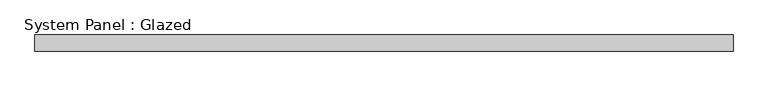
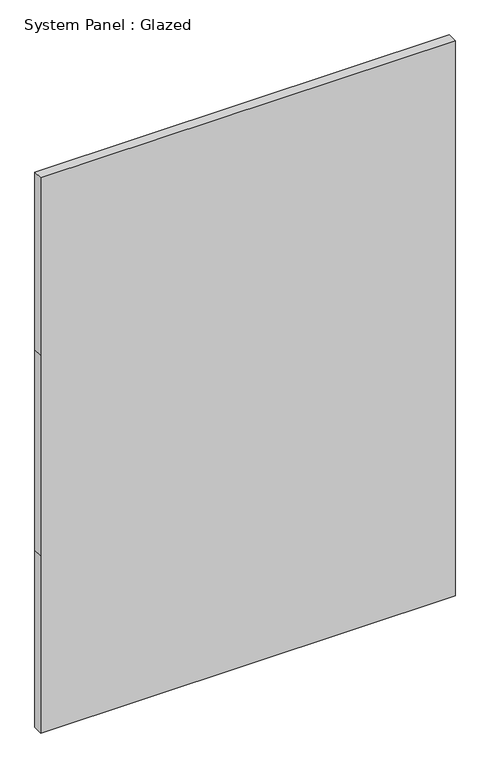
"""IFC4 building model written with IfcOpenShell, lengths in millimetres: plate geometry, System Panel : Glazed."""

from ifc_helpers import new_model, si_unit, frame, origin, place, context, project, spatial, polyline, outline, extrude, source, transform, mapped, element, save


def system_panel_glazed_ce1b7c8d(model_context):
    return source(origin(), model_context, "Body", "SweptSolid", [
        extrude(outline(polyline([(0.0, -536.575), (0.0, 536.575), (485.536674, 536.575), (1034.5733481, 536.575), (1520.1100221, 536.575), (1520.1100221, -536.575), (1034.5733481, -536.575), (485.536674, -536.575), (0.0, -536.575)])), frame((0.0, 19.05, 0.0), z_axis=(0.0, 1.0, 0.0), x_axis=(0.0, 0.0, 1.0)), (0.0, 0.0, 1.0), 25.4),
    ])


if __name__ == "__main__":
    model = new_model("IFC4")
    model_context = context("Model", 3, world=origin())
    ifc_project = project(units=[si_unit("LENGTHUNIT", "METRE", prefix="MILLI")], contexts=[model_context])
    site = spatial("IfcSite", under=ifc_project)
    building = spatial("IfcBuilding", under=site)
    placement = place(None, origin())
    system_panel_glazed_shape = system_panel_glazed_ce1b7c8d(model_context)
    element("IfcPlate", 1, ObjectType="System Panel : Glazed", at=placement, inside=building, context=model_context, shape_type="MappedRepresentation", body=[
        mapped(system_panel_glazed_shape, transform((0.0, 0.0, 0.0), x_axis=(1.0, 0.0, 0.0), y_axis=(0.0, 1.0, 0.0), z_axis=(0.0, 0.0, 1.0))),
    ])
    save(model, "model.ifc")

# Revit data of these elements
# Type "System Panel : Glazed"
#   Construction Type Id = "GSP4R"
#   Analytic Construction = "1/8 in Pilkington single glazing"
#   Visual Light Transmittance = 0.9
#   Solar Heat Gain Coefficient = 0.86
#   Heat Transfer Coefficient (U) = 1.18115 BTU/(h·ft²·°F)
#   Define Thermal Properties by = 1
# Element 1 (IfcPlate, "System Panel : Glazed")
#   Materials on its faces: "Glass"
# Materials
#   "Glass": class "Glass", colour RGB 0 128 192, transparency 0.75, Description = "Soda Lime Glass", Cost = 0
